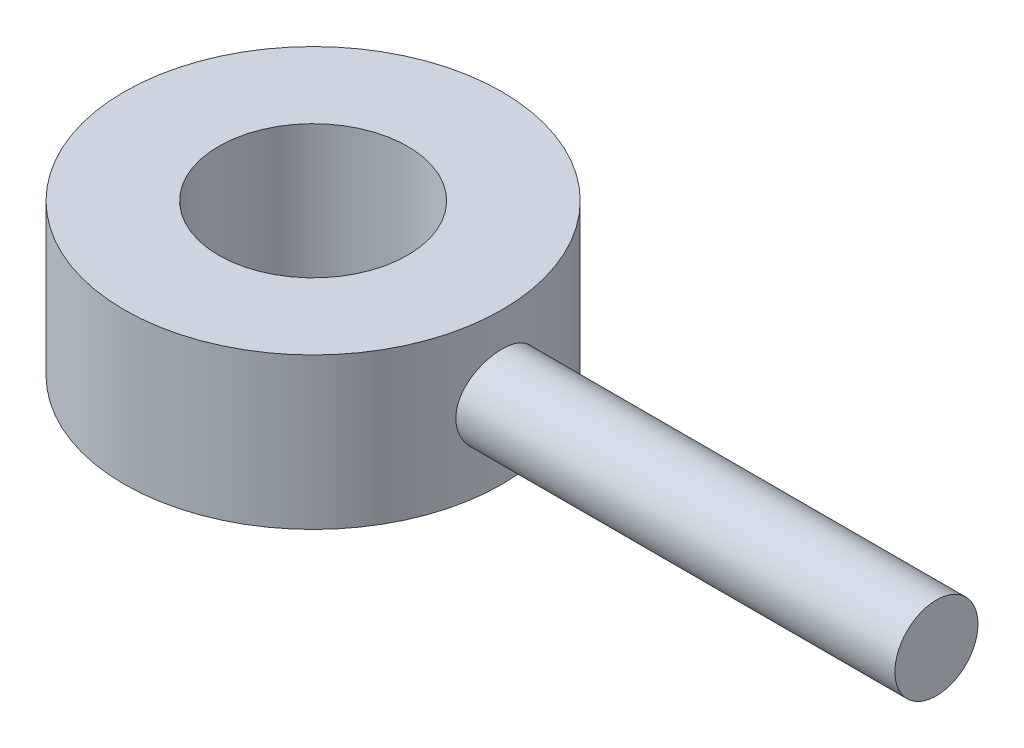
from build123d import *
from build123d.topology import SkipClean

# Parameters (mm, degrees)
HUB_RING_SKETCH_R    = 5
HUB_RING_SKETCH_R_2  = 2.5
HUB_RING_10X_5_DEPTH = 4
ARM_ROD_SKETCH_R     = 1.1
ARM_ROD_2_2_DEPTH    = 11.5
ARM_ROOT_SKETCH_R    = 1.1
ARM_ROOT_JOINT_DEPTH = 2.5


with BuildPart() as part:
    # Hub Ring Sketch → Hub Ring Ø10xØ5 (new body)
    with BuildSketch(Plane(origin=(0, 0, 0), x_dir=(1, 0, 0), z_dir=(0, 1, 0))):
        with Locations(Location((0, 0, 0), (0, 0, 270))):
            Circle(HUB_RING_SKETCH_R)
        with Locations(Location((0, 0, 0), (0, 0, 270))):
            Circle(HUB_RING_SKETCH_R_2, mode=Mode.SUBTRACT)
    extrude(amount=HUB_RING_10X_5_DEPTH)



with BuildPart() as body_2:
    # Arm Rod Sketch → Arm Rod Ø2.2 (new body)
    with BuildSketch(Plane(origin=(5, 0, 0), x_dir=(0, 0, -1), z_dir=(1, 0, 0))):
        with Locations((0, 2)):
            Circle(ARM_ROD_SKETCH_R)
    extrude(amount=ARM_ROD_2_2_DEPTH)


with BuildPart() as part_1:
    with SkipClean():  # the faces are left unmerged after this step: merging them gives an invalid solid
        add(part.part)

        add(body_2.part)  # Arm Root Joint merges body 2
        # Arm Root Sketch → Arm Root Joint (add)
        with BuildSketch(Plane(origin=(5, 0, 0), x_dir=(0, 0, -1), z_dir=(1, 0, 0))):
            with Locations((0, 2)):
                Circle(ARM_ROOT_SKETCH_R)
        extrude(amount=-ARM_ROOT_JOINT_DEPTH)


solid = part_1.part
